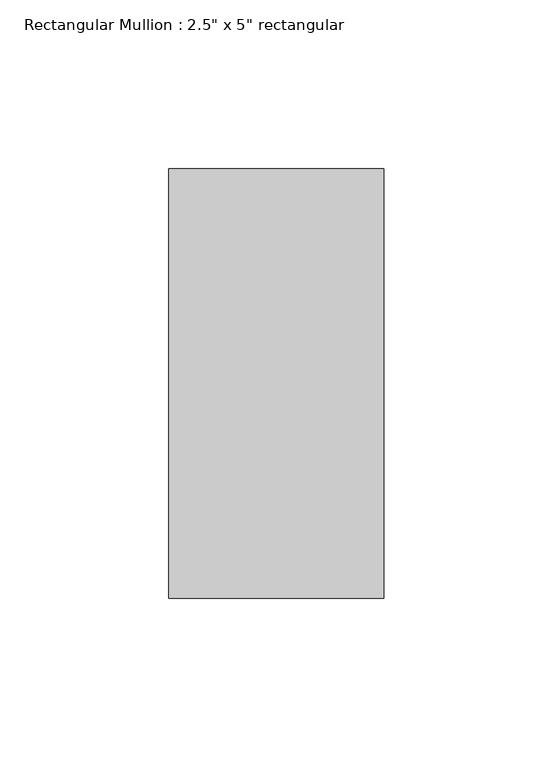
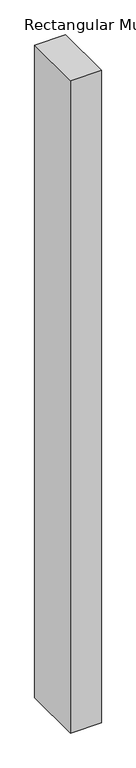
"""IFC4 building model written with IfcOpenShell, lengths in millimetres: member geometry."""

from ifc_helpers import new_model, si_unit, frame, origin, place, context, project, spatial, polyline, outline, extrude, source, transform, mapped, element, save


def member_2238a540(model_context):
    return source(origin(), model_context, "Body", "SweptSolid", [
        extrude(outline(polyline([(0.0, 63.5), (0.0, -63.5), (-63.5, -63.5), (-63.5, 63.5), (0.0, 63.5)])), frame((0.0, 0.0, -1415.4416624), z_axis=(0.0, 0.0, 1.0), x_axis=(1.0, 0.0, 0.0)), (0.0, 0.0, 1.0), 1415.4416624),
    ])


if __name__ == "__main__":
    model = new_model("IFC4")
    model_context = context("Model", 3, world=origin())
    ifc_project = project(units=[si_unit("LENGTHUNIT", "METRE", prefix="MILLI")], contexts=[model_context])
    site = spatial("IfcSite", under=ifc_project)
    building = spatial("IfcBuilding", under=site)
    placement = place(None, origin())
    member_shape = member_2238a540(model_context)
    element("IfcMember", 1, ObjectType="Rectangular Mullion : 2.5\" x 5\" rectangular", at=placement, inside=building, context=model_context, shape_type="MappedRepresentation", body=[
        mapped(member_shape, transform((0.0, 0.0, 0.0), x_axis=(1.0, 0.0, 0.0), y_axis=(0.0, 1.0, 0.0), z_axis=(0.0, 0.0, 1.0))),
    ])
    save(model, "model.ifc")

# Revit data of these elements
# Type "Rectangular Mullion : 2.5\" x 5\" rectangular"
#   built-in parameter 1007304 = 0.416667 (stored number, unit not read)
#   built-in parameter 1007301 = 0.104167 (stored number, unit not read)
#   built-in parameter 1007300 = 0.104167 (stored number, unit not read)
# Element 1 (IfcMember, "Rectangular Mullion : 2.5\" x 5\" rectangular")
#   Materials on its faces: "Aluminum"
# Materials
#   "Aluminum": class "Metal", colour RGB 247 247 247, transparency 0, Description = "Aluminum 6061", Cost = 0
